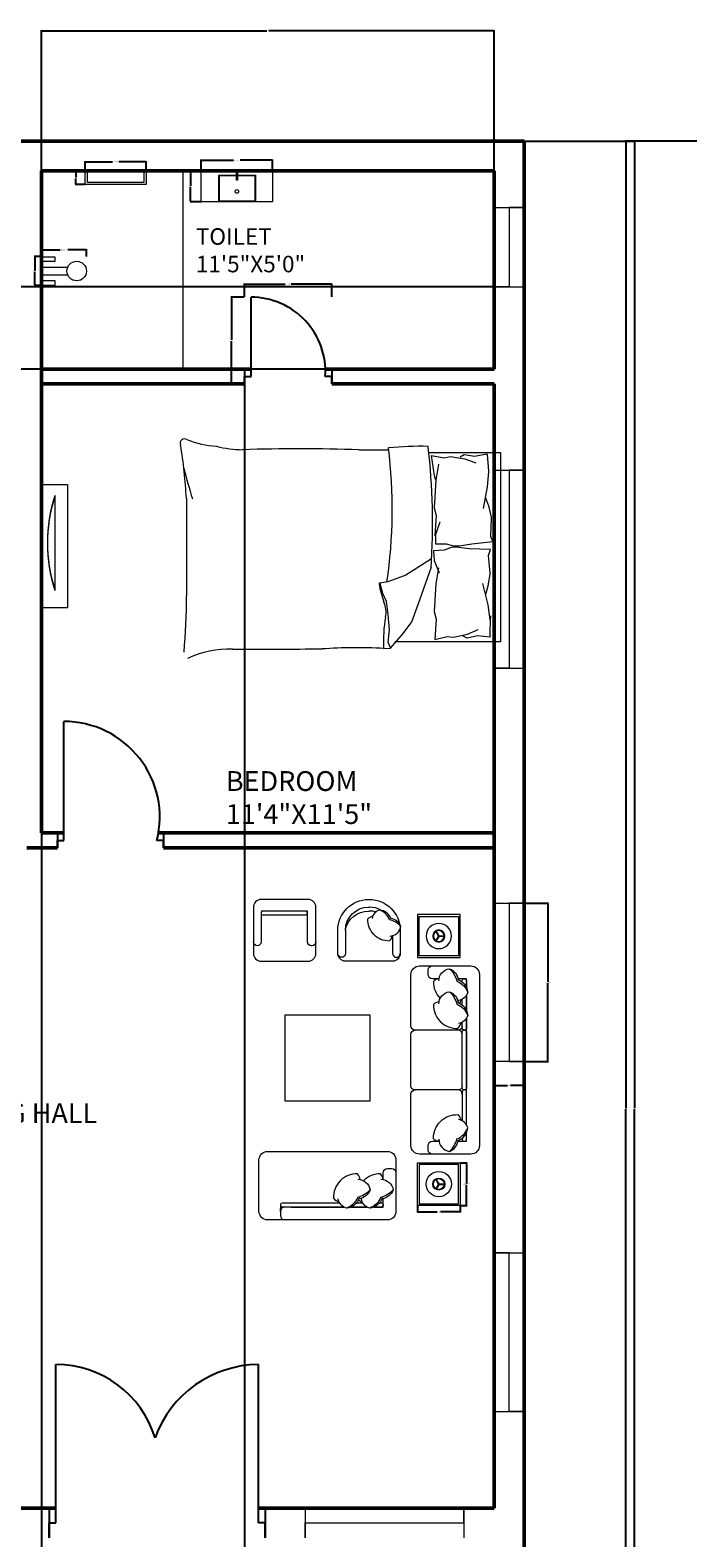
# Model space of a CAD drawing. Units: inches. Extents: x 2268 to 3372, y 1709 to 2892.
# Tile 3 of 6: x 2563 to 2762, y 2040 to 2497. Entities that reach past the tile are written whole.
import ezdxf

# ---------------------------------------------------------------- set-up
doc = ezdxf.new("R2010")
doc.units = ezdxf.units.IN
for name, color, linetype, lineweight in [('A-ANNO-DIMS', 2, 'Continuous', 18), ('A-AREA-IDEN', 7, 'Continuous', 18), ('A-DOOR', 3, 'Continuous', 25), ('A-FLOR-FIXT', 9, 'Continuous', 18), ('A-FURN', 8, 'Continuous', 18), ('A-GLAZ', 4, 'Continuous', 18), ('A-WALL', 7, 'Continuous', 50)]:
    doc.layers.add(name, color=color, linetype=linetype, lineweight=lineweight)
doc.styles.get("Standard").update_dxf_attribs({"font": 'arial.ttf'})
doc.dimstyles.get("Standard").update_dxf_attribs({"dimtxt": 0.18, "dimasz": 0.18, "dimexe": 0.18, "dimexo": 0.0625, "dimgap": 0.09, "dimtad": 0, "dimtih": 1, "dimtoh": 1, "dimdec": 4, "dimzin": 0, "dimdsep": 46, "dimtxsty": 'Standard', "dimcen": 0.09, "dimadec": 0, "dimazin": 0, "dimtfac": 1, "dimtdec": 4, "dimtofl": 0, "dimtmove": 0, "dimatfit": 3, "dimfxl": 1, "dimtolj": 1, "dimtzin": 0, "dimarcsym": 0})

# ---------------------------------------------------------------- blocks, each defined once
blk = doc.blocks.new('DOOR-ENTRY-PAIR')
for p, q in [((2, 4.5), (2, 52.5)), ((63.28, 40.5), (63.28, 52.5)), ((63.28, 4.5), (63.28, 40.5)), ((0, 9), (0, 0)), ((65.28, 9), (65.28, 0)), ((0, 0), (0, 4.5)), ((0, 4.5), (2, 4.5)), ((65.28, 4.5), (63.28, 4.5)), ((65.28, 0), (65.28, 4.5))]:
    blk.add_line(p, q)
for centre, radius, start, end in [((2, 21.15), 31.35, 16.9315, 90), ((63.59, 18.92), 33.58, 90.5202, 160.2273)]:
    blk.add_arc(centre, radius, start, end)
blk = doc.blocks.new('DOOR-BEDROOM-E')
for p, q in [((2, 2.25), (2, 38.25)), ((0, 4.5), (0, 0)), ((0, 0), (0, 2.25)), ((0, 2.25), (2, 2.25)), ((32.14, 2.25), (30.14, 2.25)), ((32.14, 4.5), (32.14, 0)), ((32.14, 0), (32.14, 2.25))]:
    blk.add_line(p, q)
blk.add_arc((2, 9.25), 29, 346.0304, 90)
blk = doc.blocks.new('DOOR-BATH-E')
for p, q in [((2, 2.25), (2, 26.25)), ((0, 4.5), (0, 0)), ((0, 0), (0, 2.25)), ((0, 2.25), (2, 2.25)), ((26.44, 2.25), (24.44, 2.25)), ((26.44, 4.5), (26.44, 0)), ((26.44, 0), (26.44, 2.25))]:
    blk.add_line(p, q)
blk.add_arc((2, 3.76), 22.49, 356.1476, 90)
blk = doc.blocks.new('WIN-48')
for p, q in [((0, 9), (0, 0)), ((48, 4.5), (48, 9)), ((48, 9), (48, 0)), ((0, 0), (0, 4.5)), ((0, 4.5), (48, 4.5))]:
    blk.add_line(p, q)
blk = doc.blocks.new('WIN-24-LONGITUDINAL')
for p, q in [((0, 24), (9, 24)), ((9, 24), (4.5, 24)), ((4.5, 24), (4.5, 0)), ((4.5, 0), (0, 0)), ((0, 0), (9, 0))]:
    blk.add_line(p, q)
blk = doc.blocks.new('WIN-60-ALTERNATE')
for p, q in [((0, 60), (9, 60)), ((9, 60), (4.5, 60)), ((4.5, 60), (4.5, 0)), ((4.5, 0), (0, 0)), ((0, 0), (9, 0))]:
    blk.add_line(p, q)
blk = doc.blocks.new('WIN-48-ALTERNATE')
for p, q in [((0, 48), (9, 48)), ((9, 48), (4.5, 48)), ((4.5, 48), (4.5, 0)), ((9, 0), (0, 0)), ((4.5, 0), (9, 0))]:
    blk.add_line(p, q)
blk = doc.blocks.new('LAVATORY-VANITY')
for points in [[(0, 9.35), (21.53, 9.35), (21.53, 0), (0, 0)], [(10.67, 8.74), (11.01, 8.74), (11.01, 6.59), (10.67, 6.59)]]:
    blk.add_lwpolyline(points, close=True)
for points in [[(11.01, 8.1), (16.38, 8.1), (16.38, 0), (5.34, 0), (5.34, 8.1), (10.67, 8.1)], [(11.01, 7.98), (16.25, 7.98), (16.25, 0.14), (5.47, 0.14), (5.47, 7.98), (10.67, 7.98)]]:
    blk.add_lwpolyline(points)
blk.add_circle((10.78, 3.14), 0.562)
blk = doc.blocks.new('SHOWER-FITTING')
for points in [[(0, 8.74), (4.04, 8.74), (4.04, 7.26), (0, 7.26)], [(0, 1.48), (4.04, 1.48), (4.04, 0), (0, 0)]]:
    blk.add_lwpolyline(points, close=True)
blk.add_lwpolyline([(7.94, 3.17), (0, 3.17), (0, 5.6), (7.94, 5.6)])
blk.add_circle((10.64, 4.38), 2.96)
blk = doc.blocks.new('SHOWER-SHELF')
for points in [[(0, 4.16), (18.51, 4.16), (18.51, 0), (0, 0)], [(0.76, 4.16), (17.78, 4.16), (17.78, 0.69), (0.76, 0.69)]]:
    blk.add_lwpolyline(points, close=True)
blk = doc.blocks.new('BEDROOM-WALL-UNIT-E')
for p, q in [((4.02, 34.02), (4.02, 5.6)), ((4.02, 33.67), (4.02, 5.25))]:
    blk.add_line(p, q)
blk.add_lwpolyline([(0, 37.37), (7.87, 37.37), (7.87, 0), (0, 0)], close=True)
for centre in [(47.85, 19.81), (47.85, 19.46)]:
    blk.add_arc(centre, 46.08, 162.0375, 197.9625)
blk = doc.blocks.new('BED-DOUBLE')
for p, q in [((0, 61.46), (31.9, 61.46)), ((0, 4.17), (0, 61.46)), ((1.84, 4.17), (1.84, 61.46)), ((3.07, 60.08), (2.95, 53.6)), ((3.07, 60.08), (6.92, 59.62)), ((6.92, 59.62), (10, 60.34)), ((14.18, 60.08), (9.9, 59.11)), ((10, 60.34), (11.25, 59.72)), ((16.11, 59.85), (14.18, 60.08)), ((19.87, 60.78), (16.11, 59.85)), ((19.38, 54.63), (19.87, 60.78)), ((33.26, 63.38), (29.37, 58.94)), ((35.36, 63.48), (33.26, 63.38, 4.64)), ((34.01, 61.54), (33.26, 63.38)), ((33.63, 57.82), (34.01, 61.54)), ((2.95, 53.6), (3.05, 54.8)), ((3.05, 54.8), (3.68, 50.25)), ((9.9, 59.11), (6.69, 57.7)), ((26.77, 55.41), (24.36, 48.73)), ((29.37, 58.94), (26.77, 55.41)), ((34.01, 53.18), (33.63, 57.82)), ((3.68, 50.25), (5.3, 43.75)), ((20.05, 52.28), (19.38, 54.63)), ((19.54, 43.87), (20.05, 52.28)), ((34.56, 49.1), (34.01, 53.18)), ((4.4, 47), (3.69, 44.52)), ((24.36, 48.73), (20.84, 38.73)), ((35.68, 46.68), (34.56, 49.1)), ((36.42, 43.71), (35.68, 46.68)), ((95, 18.06), (95, 47.57)), ((3.69, 44.52), (3.04, 41.01)), ((18.74, 39.04), (19.54, 43.87)), ((20.84, 36.28), (28.62, 41.3)), ((28.62, 41.3), (34.01, 43.34)), ((34.01, 43.34), (36.42, 43.71)), ((3.04, 41.01), (3.07, 40.62)), ((3.07, 40.62), (3.57, 35.31)), ((20.07, 36.86), (18.53, 40.55)), ((20.25, 33.92), (20.07, 36.86)), ((3.57, 35.31), (2.99, 33.54)), ((2.99, 33.54), (9.43, 33.25)), ((8.66, 31.84), (12.47, 32.54)), ((9.43, 33.25), (13.28, 32.79)), ((12.47, 32.54), (14.03, 32.54)), ((13.28, 32.79), (14.84, 32.89)), ((14.03, 32.54), (16.28, 31.84)), ((14.84, 32.89), (17.04, 33.72)), ((17.04, 33.72), (20.25, 33.92)), ((2.24, 31.15), (8.66, 31.84)), ((2.94, 29.42), (2.24, 31.15)), ((2.76, 24.09), (2.94, 29.42)), ((16.28, 31.84), (19.5, 31.84)), ((19.5, 28.9), (18.19, 25.13)), ((19.38, 23.24), (19.87, 29.39)), ((19.5, 31.84), (19.5, 28.9)), ((2.76, 23.7), (2.76, 24.09)), ((3.63, 20.23), (2.76, 23.7)), ((20.05, 20.89), (19.38, 23.24)), ((4.5, 17.81), (3.63, 20.23)), ((3.98, 14.52), (5.19, 21.1)), ((19.54, 12.48), (20.05, 20.89)), ((3.63, 9.93), (3.98, 14.52)), ((3.61, 9.81), (3.63, 9.93)), ((4, 4.67), (3.61, 9.81)), ((18.74, 7.65), (19.54, 12.48)), ((19.54, 12.48), (19.92, 11.13)), ((19.92, 11.13), (20.79, 5.02)), ((3.98, 4.67), (7.79, 5.36)), ((10.74, 6.06), (7.44, 7.27)), ((7.79, 5.36), (10.91, 4.84)), ((15.07, 5.36), (10.74, 6.06)), ((10.91, 4.84), (12.12, 5.54)), ((16.98, 5.71), (15.07, 5.36)), ((20.79, 5.02), (16.98, 5.71)), ((21.71, 4.17), (0, 4.17))]:
    blk.add_line(p, q)
for centre, radius, start, end in [((82.32, 91.3), 27.65, 267.4714, 296.4681), ((254.49, 49.33), 159.5, 174.4998, 180.6351), ((-7.98, 61.53), 43.38, 349.8763, 2.5657), ((43.54, 218.51), 155.25, 266.9791, 273.8365), ((81.31, -5405.34), 5469.02, 90.00217, 90.28689), ((42.04, 52.44), 7.46, 168.6608, 203.7384), ((1.78, 37.35), 35.55, 10.6617, 19.8806), ((187.4, 21.29), 154.68, 171.7845, 186.9006), ((36.49, 43.92), 0.221, 250.2464, 1.1377), ((218.26, 25.61), 197.77, 176.0865, 186.7821), ((-28.43, -20.65), 127.63, 13.3832, 17.7053), ((240.78, 25.69), 145.97, 182.9958, 189.4091), ((24.09, 102.1), 99.87, 268.7218, 275.604), ((37.37, -200.58), 203.94, 88.4762, 91.0082), ((60.68, 581.23), 578.22, 268.22771, 271.71854), ((77.34, -32.25), 35.53, 76.0648, 88.9113), ((84.25, -25.97), 28.25, 67.9751, 86.652), ((95.57, 1.3), 1.31, 236.1736, 23.4781)]:
    blk.add_arc(centre, radius, start, end)
blk = doc.blocks.new('LIVING-END-TABLE')
for p, q in [((6.41, 6.44), (5.49, 8.02)), ((6.41, 6.52), (5.49, 4.94)), ((6.55, 6.52), (5.63, 8.1)), ((6.55, 6.44), (5.63, 4.85)), ((6.48, 6.56), (8.3, 6.56)), ((6.48, 6.39), (8.3, 6.39))]:
    blk.add_line(p, q)
at = {"ltscale": 0.03}
blk.add_lwpolyline([(0, 0), (0, 12.95), (12.95, 12.95), (12.95, 0)], close=True, dxfattribs=at)
blk.add_lwpolyline([(0.52, 12.43), (0.52, 0.52), (12.43, 0.52), (12.43, 12.43)], close=True)
for radius in [3.82, 1.83, 1.64]:
    blk.add_circle((6.48, 6.48), radius)
blk = doc.blocks.new('*D38')
at = {"layer": 'A-ANNO-DIMS', "color": 0, "lineweight": -2, "transparency": 16777216}
for p, q in [((2628.3, 2415.99), (2628.3, 2420.07)), ((2628.48, 2419.89), (2640.59, 2419.89)), ((2654.56, 2419.89), (2642.46, 2419.89)), ((2654.74, 2415.99), (2654.74, 2420.07))]:
    blk.add_line(p, q, dxfattribs=at)
at = {"layer": 'A-ANNO-DIMS', "color": 0, "transparency": 16777216}
for points in [[(2628.48, 2419.92), (2628.48, 2419.86), (2628.3, 2419.89)], [(2654.56, 2419.92), (2654.56, 2419.86), (2654.74, 2419.89)]]:
    blk.add_solid(points, dxfattribs=at)
at = {"layer": 'Defpoints', "color": 0, "transparency": 16777216}
for p in [(2628.3, 2415.93), (2654.74, 2419.89), (2654.74, 2415.93)]:
    blk.add_point(p, dxfattribs=at)
at = {"layer": 'A-ANNO-DIMS', "color": 0, "transparency": 16777216, "insert": (2641.52, 2419.89), "char_height": 0.18, "attachment_point": 5}
blk.add_mtext('\\A1;DOOR 26 TYP.', dxfattribs=at)
blk = doc.blocks.new('*D39')
at = {"layer": 'A-ANNO-DIMS', "color": 0, "lineweight": -2, "transparency": 16777216}
for p, q in [((2628.24, 2415.93), (2624.16, 2415.93)), ((2624.34, 2415.75), (2624.34, 2402.98)), ((2624.34, 2389.86), (2624.34, 2402.62)), ((2628.24, 2389.68), (2624.16, 2389.68))]:
    blk.add_line(p, q, dxfattribs=at)
at = {"layer": 'A-ANNO-DIMS', "color": 0, "transparency": 16777216}
for points in [[(2624.31, 2415.75), (2624.37, 2415.75), (2624.34, 2415.93)], [(2624.31, 2389.86), (2624.37, 2389.86), (2624.34, 2389.68)]]:
    blk.add_solid(points, dxfattribs=at)
at = {"layer": 'Defpoints', "color": 0, "transparency": 16777216}
for p in [(2624.34, 2415.93), (2628.3, 2415.93), (2628.3, 2389.68)]:
    blk.add_point(p, dxfattribs=at)
at = {"layer": 'A-ANNO-DIMS', "color": 0, "transparency": 16777216, "insert": (2624.34, 2402.8), "char_height": 0.18, "attachment_point": 5}
blk.add_mtext('\\A1;26 TYP.', dxfattribs=at)
blk = doc.blocks.new('*D54')
at = {"layer": 'A-ANNO-DIMS', "color": 0, "lineweight": -2, "transparency": 16777216}
for p, q in [((2712.96, 2232.4), (2720.27, 2232.4)), ((2720.09, 2232.22), (2720.09, 2208.59)), ((2720.09, 2184.58), (2720.09, 2208.22)), ((2712.96, 2184.4), (2720.27, 2184.4))]:
    blk.add_line(p, q, dxfattribs=at)
at = {"layer": 'A-ANNO-DIMS', "color": 0, "transparency": 16777216}
for points in [[(2720.06, 2232.22), (2720.12, 2232.22), (2720.09, 2232.4)], [(2720.06, 2184.58), (2720.12, 2184.58), (2720.09, 2184.4)]]:
    blk.add_solid(points, dxfattribs=at)
at = {"layer": 'Defpoints', "color": 0, "transparency": 16777216}
for p in [(2712.89, 2232.4), (2720.09, 2232.4), (2712.89, 2184.4)]:
    blk.add_point(p, dxfattribs=at)
at = {"layer": 'A-ANNO-DIMS', "color": 0, "transparency": 16777216, "insert": (2720.09, 2208.4), "char_height": 0.18, "attachment_point": 5}
blk.add_mtext('\\A1;WINDOW 48 TYP.', dxfattribs=at)
blk = doc.blocks.new('*D55')
at = {"layer": 'A-ANNO-DIMS', "color": 0, "lineweight": -2, "transparency": 16777216}
for p, q in [((2703.89, 2184.34), (2703.89, 2177.02)), ((2712.89, 2184.34), (2712.89, 2177.02)), ((2704.07, 2177.2), (2707.94, 2177.2)), ((2712.71, 2177.2), (2708.85, 2177.2))]:
    blk.add_line(p, q, dxfattribs=at)
at = {"layer": 'A-ANNO-DIMS', "color": 0, "transparency": 16777216}
for points in [[(2704.07, 2177.23), (2704.07, 2177.17), (2703.89, 2177.2)], [(2712.71, 2177.23), (2712.71, 2177.17), (2712.89, 2177.2)]]:
    blk.add_solid(points, dxfattribs=at)
at = {"layer": 'Defpoints', "color": 0, "transparency": 16777216}
for p in [(2703.89, 2184.4), (2712.89, 2184.4), (2712.89, 2177.2)]:
    blk.add_point(p, dxfattribs=at)
at = {"layer": 'A-ANNO-DIMS', "color": 0, "transparency": 16777216, "insert": (2708.39, 2177.2), "char_height": 0.18, "attachment_point": 5}
blk.add_mtext('\\A1;9 TYP.', dxfattribs=at)
blk = doc.blocks.new('*D60')
at = {"layer": 'A-ANNO-DIMS', "color": 0, "lineweight": -2, "transparency": 16777216}
for p, q in [((2615.23, 2454.24), (2615.23, 2457.59)), ((2615.41, 2457.41), (2624.97, 2457.41)), ((2636.58, 2457.41), (2627.01, 2457.41)), ((2636.76, 2454.24), (2636.76, 2457.59))]:
    blk.add_line(p, q, dxfattribs=at)
at = {"layer": 'A-ANNO-DIMS', "color": 0, "transparency": 16777216}
for points in [[(2615.41, 2457.44), (2615.41, 2457.38), (2615.23, 2457.41)], [(2636.58, 2457.44), (2636.58, 2457.38), (2636.76, 2457.41)]]:
    blk.add_solid(points, dxfattribs=at)
at = {"layer": 'Defpoints', "color": 0, "transparency": 16777216}
for p in [(2636.76, 2457.41), (2615.23, 2454.18), (2636.76, 2454.18)]:
    blk.add_point(p, dxfattribs=at)
at = {"layer": 'A-ANNO-DIMS', "color": 0, "transparency": 16777216, "insert": (2625.99, 2457.41), "char_height": 0.18, "attachment_point": 5}
blk.add_mtext('\\A1;VANITY 22 TYP.', dxfattribs=at)
blk = doc.blocks.new('*D61')
at = {"layer": 'A-ANNO-DIMS', "color": 0, "lineweight": -2, "transparency": 16777216}
for p, q in [((2615.16, 2454.18), (2611.82, 2454.18)), ((2612, 2454), (2612, 2449.68)), ((2612, 2445), (2612, 2449.32)), ((2615.16, 2444.82), (2611.82, 2444.82))]:
    blk.add_line(p, q, dxfattribs=at)
at = {"layer": 'A-ANNO-DIMS', "color": 0, "transparency": 16777216}
for points in [[(2611.97, 2454), (2612.03, 2454), (2612, 2454.18)], [(2611.97, 2445), (2612.03, 2445), (2612, 2444.82)]]:
    blk.add_solid(points, dxfattribs=at)
at = {"layer": 'Defpoints', "color": 0, "transparency": 16777216}
for p in [(2612, 2454.18), (2615.23, 2454.18), (2615.23, 2444.82)]:
    blk.add_point(p, dxfattribs=at)
at = {"layer": 'A-ANNO-DIMS', "color": 0, "transparency": 16777216, "insert": (2612, 2449.5), "char_height": 0.18, "attachment_point": 5}
blk.add_mtext('\\A1;9 TYP.', dxfattribs=at)
blk = doc.blocks.new('*D62')
at = {"layer": 'A-ANNO-DIMS', "color": 0, "lineweight": -2, "transparency": 16777216}
for p, q in [((2566.89, 2428.27), (2566.89, 2430.43)), ((2567.07, 2430.25), (2572.57, 2430.25)), ((2580.32, 2430.25), (2574.82, 2430.25)), ((2580.5, 2428.27), (2580.5, 2430.43))]:
    blk.add_line(p, q, dxfattribs=at)
at = {"layer": 'A-ANNO-DIMS', "color": 0, "transparency": 16777216}
for points in [[(2567.07, 2430.28), (2567.07, 2430.22), (2566.89, 2430.25)], [(2580.32, 2430.28), (2580.32, 2430.22), (2580.5, 2430.25)]]:
    blk.add_solid(points, dxfattribs=at)
at = {"layer": 'Defpoints', "color": 0, "transparency": 16777216}
for p in [(2580.5, 2430.25), (2566.89, 2428.21), (2580.5, 2428.21)]:
    blk.add_point(p, dxfattribs=at)
at = {"layer": 'A-ANNO-DIMS', "color": 0, "transparency": 16777216, "insert": (2573.7, 2430.25), "char_height": 0.18, "attachment_point": 5}
blk.add_mtext('\\A1;SHOWER 14 TYP.', dxfattribs=at)
blk = doc.blocks.new('*D63')
at = {"layer": 'A-ANNO-DIMS', "color": 0, "lineweight": -2, "transparency": 16777216}
for p, q in [((2566.83, 2428.21), (2564.67, 2428.21)), ((2564.85, 2428.03), (2564.85, 2424.02)), ((2564.85, 2419.64), (2564.85, 2423.65)), ((2566.83, 2419.46), (2564.67, 2419.46))]:
    blk.add_line(p, q, dxfattribs=at)
at = {"layer": 'A-ANNO-DIMS', "color": 0, "transparency": 16777216}
for points in [[(2564.82, 2428.03), (2564.88, 2428.03), (2564.85, 2428.21)], [(2564.82, 2419.64), (2564.88, 2419.64), (2564.85, 2419.46)]]:
    blk.add_solid(points, dxfattribs=at)
at = {"layer": 'Defpoints', "color": 0, "transparency": 16777216}
for p in [(2564.85, 2428.21), (2566.89, 2428.21), (2566.89, 2419.46)]:
    blk.add_point(p, dxfattribs=at)
at = {"layer": 'A-ANNO-DIMS', "color": 0, "transparency": 16777216, "insert": (2564.85, 2423.83), "char_height": 0.18, "attachment_point": 5}
blk.add_mtext('\\A1;9 TYP.', dxfattribs=at)
blk = doc.blocks.new('*D64')
at = {"layer": 'A-ANNO-DIMS', "color": 0, "lineweight": -2, "transparency": 16777216}
for p, q in [((2580.05, 2454.24), (2580.05, 2457.13)), ((2580.23, 2456.95), (2588.34, 2456.95)), ((2598.39, 2456.95), (2590.28, 2456.95)), ((2598.57, 2454.24), (2598.57, 2457.13))]:
    blk.add_line(p, q, dxfattribs=at)
at = {"layer": 'A-ANNO-DIMS', "color": 0, "transparency": 16777216}
for points in [[(2580.23, 2456.98), (2580.23, 2456.92), (2580.05, 2456.95)], [(2598.39, 2456.98), (2598.39, 2456.92), (2598.57, 2456.95)]]:
    blk.add_solid(points, dxfattribs=at)
at = {"layer": 'Defpoints', "color": 0, "transparency": 16777216}
for p in [(2598.57, 2456.95), (2580.05, 2454.18), (2598.57, 2454.18)]:
    blk.add_point(p, dxfattribs=at)
at = {"layer": 'A-ANNO-DIMS', "color": 0, "transparency": 16777216, "insert": (2589.31, 2456.95), "char_height": 0.18, "attachment_point": 5}
blk.add_mtext('\\A1;SHELF 19 TYP.', dxfattribs=at)
blk = doc.blocks.new('*D65')
at = {"layer": 'A-ANNO-DIMS', "color": 0, "lineweight": -2, "transparency": 16777216}
for p, q in [((2579.99, 2454.18), (2577.09, 2454.18)), ((2577.27, 2454), (2577.27, 2452.28)), ((2579.99, 2450.02), (2577.09, 2450.02)), ((2577.27, 2450.2), (2577.27, 2451.92))]:
    blk.add_line(p, q, dxfattribs=at)
at = {"layer": 'A-ANNO-DIMS', "color": 0, "transparency": 16777216}
for points in [[(2577.24, 2454), (2577.3, 2454), (2577.27, 2454.18)], [(2577.24, 2450.2), (2577.3, 2450.2), (2577.27, 2450.02)]]:
    blk.add_solid(points, dxfattribs=at)
at = {"layer": 'Defpoints', "color": 0, "transparency": 16777216}
for p in [(2577.27, 2454.18), (2580.05, 2454.18), (2580.05, 2450.02)]:
    blk.add_point(p, dxfattribs=at)
at = {"layer": 'A-ANNO-DIMS', "color": 0, "transparency": 16777216, "insert": (2577.27, 2452.1), "char_height": 0.18, "attachment_point": 5}
blk.add_mtext('\\A1;4 TYP.', dxfattribs=at)
blk = doc.blocks.new('*D72')
at = {"layer": 'A-ANNO-DIMS', "color": 0, "lineweight": -2, "transparency": 16777216}
for p, q in [((2693.64, 2153.8), (2695.7, 2153.8)), ((2695.52, 2153.62), (2695.52, 2147.5)), ((2695.52, 2141.02), (2695.52, 2147.14)), ((2693.64, 2140.84), (2695.7, 2140.84))]:
    blk.add_line(p, q, dxfattribs=at)
at = {"layer": 'A-ANNO-DIMS', "color": 0, "transparency": 16777216}
for points in [[(2695.49, 2153.62), (2695.55, 2153.62), (2695.52, 2153.8)], [(2695.49, 2141.02), (2695.55, 2141.02), (2695.52, 2140.84)]]:
    blk.add_solid(points, dxfattribs=at)
at = {"layer": 'Defpoints', "color": 0, "transparency": 16777216}
for p in [(2693.58, 2153.8), (2695.52, 2153.8), (2693.58, 2140.84)]:
    blk.add_point(p, dxfattribs=at)
at = {"layer": 'A-ANNO-DIMS', "color": 0, "transparency": 16777216, "insert": (2695.52, 2147.32), "char_height": 0.18, "attachment_point": 5}
blk.add_mtext('\\A1;END TABLE 13 TYP.', dxfattribs=at)
blk = doc.blocks.new('*D73')
at = {"layer": 'A-ANNO-DIMS', "color": 0, "lineweight": -2, "transparency": 16777216}
for p, q in [((2680.63, 2140.78), (2680.63, 2138.72)), ((2680.81, 2138.9), (2686.58, 2138.9)), ((2693.4, 2138.9), (2687.62, 2138.9)), ((2693.58, 2140.78), (2693.58, 2138.72))]:
    blk.add_line(p, q, dxfattribs=at)
at = {"layer": 'A-ANNO-DIMS', "color": 0, "transparency": 16777216}
for points in [[(2680.81, 2138.93), (2680.81, 2138.87), (2680.63, 2138.9)], [(2693.4, 2138.93), (2693.4, 2138.87), (2693.58, 2138.9)]]:
    blk.add_solid(points, dxfattribs=at)
at = {"layer": 'Defpoints', "color": 0, "transparency": 16777216}
for p in [(2680.63, 2140.84), (2693.58, 2140.84), (2693.58, 2138.9)]:
    blk.add_point(p, dxfattribs=at)
at = {"layer": 'A-ANNO-DIMS', "color": 0, "transparency": 16777216, "insert": (2687.1, 2138.9), "char_height": 0.18, "attachment_point": 5}
blk.add_mtext('\\A1;13 TYP.', dxfattribs=at)
blk = doc.blocks.new('*D77')
at = {"layer": 'A-ANNO-DIMS', "color": 0, "lineweight": -2, "transparency": 16777216}
for p, q in [((2712.96, 2463.18), (2746.52, 2463.18)), ((2746.34, 2463), (2746.34, 2170.36)), ((2746.34, 1877.36), (2746.34, 2169.99)), ((2712.96, 1877.18), (2746.52, 1877.18))]:
    blk.add_line(p, q, dxfattribs=at)
at = {"layer": 'A-ANNO-DIMS', "color": 0, "transparency": 16777216}
for points in [[(2746.31, 2463), (2746.37, 2463), (2746.34, 2463.18)], [(2746.31, 1877.36), (2746.37, 1877.36), (2746.34, 1877.18)]]:
    blk.add_solid(points, dxfattribs=at)
at = {"layer": 'Defpoints', "color": 0, "transparency": 16777216}
for p in [(2712.89, 2463.18), (2746.34, 2463.18), (2712.89, 1877.18)]:
    blk.add_point(p, dxfattribs=at)
at = {"layer": 'A-ANNO-DIMS', "color": 0, "transparency": 16777216, "insert": (2746.34, 2170.18), "char_height": 0.18, "attachment_point": 5}
blk.add_mtext('\\A1;586', dxfattribs=at)
blk = doc.blocks.new('*D80')
at = {"layer": 'A-ANNO-DIMS', "color": 0, "lineweight": -2, "transparency": 16777216}
for p, q in [((2566.89, 2454.24), (2566.89, 2496.81)), ((2567.07, 2496.63), (2635.11, 2496.63)), ((2703.71, 2496.63), (2635.67, 2496.63)), ((2703.89, 2454.24), (2703.89, 2496.81))]:
    blk.add_line(p, q, dxfattribs=at)
at = {"layer": 'A-ANNO-DIMS', "color": 0, "transparency": 16777216}
for points in [[(2567.07, 2496.66), (2567.07, 2496.6), (2566.89, 2496.63)], [(2703.71, 2496.66), (2703.71, 2496.6), (2703.89, 2496.63)]]:
    blk.add_solid(points, dxfattribs=at)
at = {"layer": 'Defpoints', "color": 0, "transparency": 16777216}
for p in [(2703.89, 2496.63), (2566.89, 2454.18), (2703.89, 2454.18)]:
    blk.add_point(p, dxfattribs=at)
at = {"layer": 'A-ANNO-DIMS', "color": 0, "transparency": 16777216, "insert": (2635.39, 2496.63), "char_height": 0.18, "attachment_point": 5}
blk.add_mtext('\\A1;137', dxfattribs=at)
blk = doc.blocks.new('*D82')
at = {"layer": 'A-ANNO-DIMS', "color": 0, "lineweight": -2, "transparency": 16777216}
for p, q in [((2566.89, 2389.61), (2566.89, 1790.27)), ((2628.3, 2389.61), (2628.3, 1790.27)), ((2567.07, 1790.45), (2597.22, 1790.45)), ((2628.12, 1790.45), (2597.98, 1790.45))]:
    blk.add_line(p, q, dxfattribs=at)
at = {"layer": 'A-ANNO-DIMS', "color": 0, "transparency": 16777216}
for points in [[(2567.07, 1790.48), (2567.07, 1790.42), (2566.89, 1790.45)], [(2628.12, 1790.48), (2628.12, 1790.42), (2628.3, 1790.45)]]:
    blk.add_solid(points, dxfattribs=at)
at = {"layer": 'Defpoints', "color": 0, "transparency": 16777216}
for p in [(2566.89, 2389.68), (2628.3, 2389.68), (2628.3, 1790.45)]:
    blk.add_point(p, dxfattribs=at)
at = {"layer": 'A-ANNO-DIMS', "color": 0, "transparency": 16777216, "insert": (2597.6, 1790.45), "char_height": 0.18, "attachment_point": 5}
blk.add_mtext('\\A1;61.41', dxfattribs=at)
blk = doc.blocks.new('*D93')
at = {"layer": 'A-ANNO-DIMS', "color": 0, "lineweight": -2, "transparency": 16777216}
for p, q in [((2812.94, 2463.18), (2743.52, 2463.18)), ((2743.7, 2463), (2743.7, 2170.36)), ((2743.7, 1877.36), (2743.7, 2169.99)), ((2812.94, 1877.18), (2743.52, 1877.18))]:
    blk.add_line(p, q, dxfattribs=at)
at = {"layer": 'A-ANNO-DIMS', "color": 0, "transparency": 16777216}
for points in [[(2743.67, 2463), (2743.73, 2463), (2743.7, 2463.18)], [(2743.67, 1877.36), (2743.73, 1877.36), (2743.7, 1877.18)]]:
    blk.add_solid(points, dxfattribs=at)
at = {"layer": 'Defpoints', "color": 0, "transparency": 16777216}
for p in [(2743.7, 2463.18), (2813, 2463.18), (2813, 1877.18)]:
    blk.add_point(p, dxfattribs=at)
at = {"layer": 'A-ANNO-DIMS', "color": 0, "transparency": 16777216, "insert": (2743.7, 2170.18), "char_height": 0.18, "attachment_point": 5}
blk.add_mtext('\\A1;586', dxfattribs=at)
blk = doc.blocks.new('*D98')
at = {"layer": 'A-ANNO-DIMS', "color": 0, "lineweight": -2, "transparency": 16777216}
for p, q in [((2703.83, 2419.05), (2329.26, 2419.05)), ((2329.44, 2418.87), (2329.44, 2406.8)), ((2329.44, 2394.36), (2329.44, 2406.43)), ((2703.83, 2394.18), (2329.26, 2394.18))]:
    blk.add_line(p, q, dxfattribs=at)
at = {"layer": 'A-ANNO-DIMS', "color": 0, "transparency": 16777216}
for points in [[(2329.41, 2418.87), (2329.47, 2418.87), (2329.44, 2419.05)], [(2329.41, 2394.36), (2329.47, 2394.36), (2329.44, 2394.18)]]:
    blk.add_solid(points, dxfattribs=at)
at = {"layer": 'Defpoints', "color": 0, "transparency": 16777216}
for p in [(2329.44, 2419.05), (2703.89, 2419.05), (2703.89, 2394.18)]:
    blk.add_point(p, dxfattribs=at)
at = {"layer": 'A-ANNO-DIMS', "color": 0, "transparency": 16777216, "insert": (2329.44, 2406.61), "char_height": 0.18, "attachment_point": 5}
blk.add_mtext('\\A1;24.88', dxfattribs=at)

msp = doc.modelspace()

# ---------------------------------------------------------------- linework, layer by layer
at = {"layer": 'A-FLOR-FIXT'}
msp.add_line((2609.6995, 2454.1756), (2609.6995, 2394.1756), dxfattribs=at)
msp.add_line((2609.6995, 2454.1756), (2609.6995, 2394.1756), dxfattribs=at)
at = {"layer": 'A-FURN'}
msp.add_line((2639.1743, 2139.0646), (2639.3001, 2141.0076), dxfattribs=at)
at = {"layer": 'A-FURN', "ltscale": 0.03}
for points in [[(2633.3396, 2233.5207), (2633.3396, 2233.5207, 0.41421356), (2631.0037, 2231.1848), (2631.0037, 2217.1696, 0.41421356), (2633.3396, 2214.8337), (2633.3396, 2214.8337), (2647.5885, 2214.8337, 0.41421356), (2649.9244, 2217.1696), (2649.9244, 2231.1848, 0.41421356), (2647.5885, 2233.5207)], [(2681.2733, 2156.3858, -0.41421356), (2678.6826, 2158.9765), (2678.6826, 2174.5207, -0.41421356), (2679.9779, 2175.816, -0.41421356), (2678.6826, 2177.1114), (2678.6826, 2192.6556, -0.41421356), (2679.9779, 2193.951, -0.41421356), (2678.6826, 2195.2463), (2678.6826, 2210.7905, -0.41421356), (2681.2733, 2213.3812), (2696.8175, 2213.3812, -0.41421356), (2699.4082, 2210.7905), (2699.4082, 2158.9765, -0.41421356), (2696.8175, 2156.3858)], [(2632.6976, 2154.6088, -0.41421356), (2635.2883, 2157.1995), (2635.2883, 2157.1995, 0.31783725), (2635.2883, 2157.1995, -0.41421356), (2635.2883, 2157.1995), (2635.2883, 2157.1995, 1.18618475), (2635.2883, 2157.1995, -0.41421356), (2635.2883, 2157.1995), (2671.5581, 2157.1995, -0.41421356), (2674.1488, 2154.6088), (2674.1488, 2139.0646, -0.41421356), (2671.5581, 2136.4739), (2635.2883, 2136.4739, -0.41421356), (2632.6976, 2139.0646)]]:
    msp.add_lwpolyline(points, format="xyb", close=True, dxfattribs=at)
msp.add_lwpolyline([(2665.9881, 2214.8337), (2658.8637, 2214.8337, -0.41421356), (2656.5278, 2217.1696), (2656.5278, 2224.1772, -0.41421356), (2665.8713, 2233.5207), (2665.9881, 2233.5207), (2666.1049, 2233.5207, -0.41421356), (2675.4484, 2224.1772), (2675.4484, 2217.1696, -0.41421356), (2673.1126, 2214.8337), (2665.9881, 2214.8337)], format="xyb", dxfattribs=at)
at = {"layer": 'A-FURN'}
for points in [[(2633.3396, 2229.3161), (2633.3396, 2220.6734, -0.41421356), (2632.1717, 2219.5054), (2632.1717, 2219.5054, -0.41421356), (2631.0037, 2220.6734)], [(2642.9548, 2230.0169), (2633.8068, 2230.0169, 0.41421356), (2633.3396, 2229.5497), (2633.3396, 2229.3161, 0.41421356), (2633.8068, 2228.849), (2641.7788, 2228.849, 0.41421356)], [(2641.7788, 2228.849), (2646.8877, 2228.849, 0.41421356), (2647.3549, 2229.3161), (2647.3549, 2229.5497, 0.41421356), (2646.8877, 2230.0169)], [(2646.8877, 2230.0169), (2642.9548, 2230.0169, 0.41421356)], [(2658.8637, 2224.1772, -0.41421356), (2665.8713, 2231.1848), (2665.9881, 2231.1848)], [(2658.8637, 2224.1772, -0.37271891), (2665.8713, 2230.0169), (2665.9881, 2230.0169)], [(2672.8815, 2222.4835, -0.16554063), (2672.159, 2220.9403, -0.42598917), (2665.5996, 2227.631, -0.12152332), (2667.1567, 2228.5532, 7.11546429)], [(2669.5834, 2230.2606, 0.13059149), (2666.1049, 2231.1848), (2665.9881, 2231.1848)], [(2668.0962, 2229.7652, 0.07238424), (2666.1049, 2230.0169), (2665.9881, 2230.0169)], [(2672.6975, 2227.5234, 0.30666349), (2669.214, 2230.3073, 0.30632997), (2666.9383, 2227.7649, -0.87284716)], [(2675.6395, 2225.3562, 0.14772988), (2672.2259, 2227.3634, 0.21334276), (2669.214, 2230.3073, 0.17866181)], [(2658.8637, 2224.1773), (2658.8637, 2217.1696, -0.41421356), (2657.6958, 2216.0016), (2657.6958, 2216.0016, -0.41421356), (2656.5278, 2217.1696)], [(2672.2929, 2222.4123, 0.35677236), (2675.6395, 2225.3562, 0.24954205), (2672.6071, 2227.7822, -9.61688035)], [(2649.9244, 2220.6734, -0.41421356), (2648.7564, 2219.5054), (2648.5228, 2219.5054, -0.41421356), (2647.3549, 2220.6734), (2647.3549, 2222.4829)], [(2673.1126, 2222.5396), (2673.1126, 2217.1696, 0.41421356), (2674.2805, 2216.0016), (2674.2805, 2216.0016, 0.41421356), (2675.4484, 2217.1696)], [(2687.1663, 2209.4952), (2685.1593, 2209.4952, -0.41421356), (2683.864, 2210.7905), (2683.864, 2212.0859, -0.41421356), (2685.1593, 2213.3812)], [(2687.0879, 2208.8451, -0.35677236), (2690.353, 2212.5568, -0.24954205), (2693.0437, 2209.1937)], [(2690.353, 2212.5568, -0.14772988), (2692.5792, 2208.7709, -0.21334276), (2695.8443, 2205.4304)], [(2687.1669, 2209.498, 0.16554063), (2685.4554, 2208.6967, 0.20023115), (2687.5398, 2203.5546)], [(2687.0879, 2201.8671, -0.35677236), (2690.353, 2205.5788, -0.24954205), (2693.0437, 2202.2157)], [(2690.353, 2205.5788, -0.14772988), (2692.5792, 2201.7929, -0.21334276), (2695.8443, 2198.4523)], [(2692.7566, 2209.2939, -0.30666349), (2695.8443, 2205.4304, -0.30632997), (2693.0244, 2202.9064)], [(2695.5222, 2206.7701), (2695.5222, 2209.4952), (2692.9765, 2209.4952, -0.41435211)], [(2694.2268, 2208.5067), (2694.2268, 2208.977, -0.41421356), (2694.7449, 2209.4952), (2695.004, 2209.4952, -0.41421356), (2695.5222, 2208.977)], [(2695.5222, 2208.977), (2695.5222, 2206.7701, -0.41446868)], [(2687.1669, 2202.52, 0.16554063), (2685.4554, 2201.7187, 0.42598917), (2692.876, 2194.4437, 0.12152332), (2693.8988, 2196.1706)], [(2692.7566, 2202.3159, -0.30666349), (2695.8443, 2198.4523, -0.30632997), (2693.0244, 2195.9284)], [(2693.3924, 2202.0626, 0.07186538), (2693.8988, 2203.1486)], [(2694.2268, 2201.5287), (2694.2268, 2203.3108, -0.41459885)], [(2695.5222, 2204.6151), (2695.5222, 2199.7921, -0.41474665)], [(2695.5222, 2197.6371), (2695.5222, 2194.4691, -0.41421356), (2695.004, 2193.951), (2694.7449, 2193.951, -0.41421356), (2694.2268, 2194.4691), (2694.2268, 2196.3328, -0.12631336)], [(2694.2268, 2195.2463, -0.41421356), (2692.9314, 2193.951), (2679.9779, 2193.951, -0.41732018)], [(2694.2268, 2192.6556, 0.41421356), (2692.9314, 2193.951)], [(2694.2268, 2174.5207, 0.41421356), (2692.9314, 2175.816), (2679.9779, 2175.816, 0.4152491)], [(2694.2268, 2177.1114, -0.41421356), (2692.9314, 2175.816)], [(2695.5222, 2165.1519), (2695.5222, 2175.2979, 0.41421356), (2695.004, 2175.816), (2694.7449, 2175.816, 0.41421356), (2694.2268, 2175.2979), (2694.2268, 2166.4562, 0.41265155)], [(2687.1669, 2160.269, -0.16554063), (2685.4554, 2161.0703, -0.42598917), (2692.876, 2168.3453, -0.12152332), (2693.8988, 2166.6184)], [(2692.7566, 2160.4731, 0.30666349), (2695.8443, 2164.3366, 0.30632997), (2693.0244, 2166.8606)], [(2685.1593, 2156.3858, -0.41421356), (2683.864, 2157.6811), (2683.864, 2158.9765, -0.41421356), (2685.1593, 2160.2718), (2687.1663, 2160.2718)], [(2687.0879, 2160.9219, 0.35677236), (2690.353, 2157.2102, 0.24954205), (2693.0437, 2160.5733)], [(2690.353, 2157.2102, 0.14772988), (2692.5792, 2160.9961, 0.21334276), (2695.8443, 2164.3366)], [(2694.2268, 2161.2603), (2694.2268, 2160.79, 0.41421356), (2694.7449, 2160.2718), (2695.004, 2160.2718, 0.41421356), (2695.5222, 2160.79)], [(2695.5222, 2160.79), (2695.5222, 2162.9969, 0.41253535)], [(2670.2628, 2148.7158), (2670.2628, 2150.7227, -0.41421356), (2671.5581, 2152.0181), (2672.8535, 2152.0181, -0.41421356), (2674.1488, 2150.7227)], [(2663.2876, 2148.7152, 0.16554063), (2662.4862, 2150.4267, 0.42598917), (2655.2113, 2143.0061, 0.12152332), (2656.9382, 2141.9832, -7.11546429)], [(2662.6347, 2148.7942, -0.35677236), (2666.3464, 2145.5291, -0.24954205), (2662.9833, 2142.8384, 9.61688035)], [(2670.2656, 2148.7152, 0.16554063), (2669.4643, 2150.4267, 0.20023115), (2664.3222, 2148.3422, 0.12152332)], [(2669.6127, 2148.7942, -0.35677236), (2673.3244, 2145.5291, -0.24954205), (2669.9613, 2142.8384, 9.61688035)], [(2658.4047, 2140.3599), (2639.8183, 2140.3599, -0.41421356), (2639.3001, 2140.8781), (2639.3001, 2141.1371, -0.41421356), (2639.8183, 2141.6553), (2657.1004, 2141.6553, -0.41421356)], [(2663.0835, 2143.1255, -0.30666349), (2659.2199, 2140.0378, -0.30632997), (2656.696, 2142.8576, 0.87284716)], [(2666.3464, 2145.5291, -0.14772988), (2662.5605, 2143.3029, -0.21334276), (2659.2199, 2140.0378, -0.17866181)], [(2662.2963, 2141.6553), (2664.0784, 2141.6553, -0.41421356)], [(2662.8302, 2142.4897, 0.07186538), (2663.9162, 2141.9832, -7.11546429)], [(2670.0615, 2143.1255, -0.30666349), (2666.198, 2140.0378, -0.30632997), (2663.674, 2142.8576, 0.87284716)], [(2673.3244, 2145.5291, -0.14772988), (2669.5385, 2143.3029, -0.21334276), (2666.198, 2140.0378, -0.17866181)], [(2667.5377, 2140.3599), (2670.2628, 2140.3599), (2670.2628, 2142.9056, -0.41421356)], [(2669.2743, 2141.6553), (2669.7446, 2141.6553, -0.41421356), (2670.2628, 2141.1371), (2670.2628, 2140.8781, -0.41421356), (2669.7446, 2140.3599)], [(2642.4767, 2140.3599), (2640.4697, 2140.3599, 0.41421356), (2639.1743, 2139.0646), (2639.1743, 2137.7692, 0.41421356), (2640.4697, 2136.4739)], [(2665.3827, 2140.3599), (2660.5597, 2140.3599, -0.41421356)], [(2669.7446, 2140.3599), (2667.5377, 2140.3599, -0.41421356)]]:
    msp.add_lwpolyline(points, format="xyb", dxfattribs=at)
for points in [[(2642.9548, 2230.0169), (2633.4564, 2230.0169)], [(2647.3549, 2222.4829), (2647.3549, 2230.0169), (2642.9548, 2230.0169)], [(2695.5222, 2199.7921), (2695.5222, 2204.6151)], [(2695.5222, 2165.1519), (2695.5222, 2197.6371)], [(2692.9765, 2160.2718), (2695.5222, 2160.2718), (2695.5222, 2162.9969)], [(2642.4767, 2140.3599), (2658.4047, 2140.3599)], [(2660.5597, 2140.3599), (2665.3827, 2140.3599)]]:
    msp.add_lwpolyline(points, dxfattribs=at)
at = {"layer": 'A-FURN', "ltscale": 0.03}
msp.add_lwpolyline([(2640.4697, 2198.4847), (2640.4697, 2172.5777), (2666.3767, 2172.5777), (2666.3767, 2198.4847)], close=True, dxfattribs=at)
at = {"layer": 'A-FURN'}
msp.add_lwpolyline([(2695.5222, 2193.4328), (2695.5222, 2176.3342, -0.41421356), (2695.004, 2175.816), (2694.7449, 2175.816, -0.41421356), (2694.2268, 2176.3342), (2694.2268, 2193.4328, -0.41421356), (2694.7449, 2193.951), (2695.004, 2193.951, -0.41421356)], format="xyb", close=True, dxfattribs=at)
at = {"layer": 'A-WALL'}
for p, q in [((2362.8943, 2463.1756), (2712.8943, 2463.1756)), ((2362.8943, 2463.1756), (2712.8943, 2463.1756)), ((2362.8943, 2463.1756), (2712.8943, 2463.1756)), ((2362.8943, 2463.1756), (2712.8943, 2463.1756)), ((2712.8943, 2463.1756), (2712.8943, 1877.1756)), ((2712.8943, 2463.1756), (2712.8943, 1877.1756)), ((2566.8943, 2454.1756), (2566.8943, 2253.6756)), ((2566.8943, 2454.1756), (2703.8943, 2454.1756)), ((2566.8943, 2454.1756), (2703.8943, 2454.1756)), ((2566.8943, 2454.1756), (2566.8943, 2253.6756)), ((2703.8943, 2454.1756), (2703.8943, 2394.1756)), ((2703.8943, 2454.1756), (2703.8943, 2394.1756)), ((2566.8943, 2394.1756), (2630.3027, 2394.1756)), ((2566.8943, 2394.1756), (2630.3027, 2394.1756)), ((2652.7796, 2394.1756), (2703.8943, 2394.1756)), ((2652.7796, 2394.1756), (2703.8943, 2394.1756)), ((2566.8943, 2389.6756), (2628.3027, 2389.6756)), ((2566.8943, 2389.6756), (2628.3027, 2389.6756)), ((2654.7409, 2389.6756), (2703.8943, 2389.6756)), ((2654.7409, 2389.6756), (2703.8943, 2389.6756)), ((2703.8943, 2389.6756), (2703.8943, 2049.1756)), ((2703.8943, 2389.6756), (2703.8943, 2049.1756)), ((2566.8943, 2253.6756), (2573.6791, 2253.6756)), ((2566.8943, 2253.6756), (2573.6791, 2253.6756)), ((2602.2867, 2253.6756), (2703.8943, 2253.6756)), ((2602.2867, 2253.6756), (2703.8943, 2253.6756)), ((2566.8943, 2249.1756), (2562.3943, 2249.1756)), ((2566.8943, 2249.1756), (2562.3943, 2249.1756)), ((2566.8943, 2249.1756), (2571.6791, 2249.1756)), ((2566.8943, 2249.1756), (2571.6791, 2249.1756)), ((2603.8208, 2249.1756), (2703.8943, 2249.1756)), ((2603.8208, 2249.1756), (2703.8943, 2249.1756)), ((2496.3943, 2049.1756), (2571.2467, 2049.1756)), ((2496.3943, 2049.1756), (2571.2467, 2049.1756)), ((2632.5318, 2049.1756), (2703.8943, 2049.1756)), ((2632.5318, 2049.1756), (2703.8943, 2049.1756))]:
    msp.add_line(p, q, dxfattribs=at)

# ---------------------------------------------------------------- block references
at = {"layer": 'A-DOOR'}
for name, p in [('DOOR-BATH-E', (2628.303, 2389.676)), ('DOOR-BATH-E', (2628.303, 2389.676)), ('DOOR-BEDROOM-E', (2571.679, 2249.176)), ('DOOR-BEDROOM-E', (2571.679, 2249.176)), ('DOOR-ENTRY-PAIR', (2569.247, 2040.176)), ('DOOR-ENTRY-PAIR', (2569.247, 2040.176))]:
    msp.add_blockref(name, p, dxfattribs=at)
at = {"layer": 'A-FLOR-FIXT'}
for name, p in [('SHOWER-SHELF', (2580.052, 2450.016)), ('SHOWER-SHELF', (2580.052, 2450.016)), ('LAVATORY-VANITY', (2615.227, 2444.822)), ('LAVATORY-VANITY', (2615.227, 2444.822)), ('SHOWER-FITTING', (2566.894, 2419.462)), ('SHOWER-FITTING', (2566.894, 2419.462))]:
    msp.add_blockref(name, p, dxfattribs=at)
at = {"layer": 'A-FURN', "rotation": 180}
msp.add_blockref('BED-DOUBLE', (2705.7331, 2373.0128), dxfattribs=at)
at = {"layer": 'A-FURN'}
for name, p in [('BEDROOM-WALL-UNIT-E', (2566.894, 2321.841)), ('BEDROOM-WALL-UNIT-E', (2566.894, 2321.841)), ('LIVING-END-TABLE', (2680.626, 2140.842))]:
    msp.add_blockref(name, p, dxfattribs=at)
at = {"layer": 'A-FURN', "extrusion": (0, 0, -1), "zscale": -1, "rotation": 180}
msp.add_blockref('LIVING-END-TABLE', (-2680.626, 2228.925), dxfattribs=at)
at = {"layer": 'A-GLAZ'}
for name, p in [('WIN-24-LONGITUDINAL', (2703.894, 2419.053)), ('WIN-24-LONGITUDINAL', (2703.894, 2419.053)), ('WIN-60-ALTERNATE', (2703.894, 2303.531)), ('WIN-60-ALTERNATE', (2703.894, 2303.531)), ('WIN-48-ALTERNATE', (2703.894, 2184.405)), ('WIN-48-ALTERNATE', (2703.894, 2184.405)), ('WIN-48', (2646.685, 2040.176)), ('WIN-48', (2646.685, 2040.176))]:
    msp.add_blockref(name, p, dxfattribs=at)
for rotation in [89.9999999999993, 89.99999999999739]:
    msp.add_blockref('WIN-48', (2712.8939, 2078.4469), dxfattribs=dict(at, rotation=rotation))

# ---------------------------------------------------------------- texts
at = {"layer": 'A-AREA-IDEN', "attachment_point": 1}
for s, width, insert, char_height in [('TOILET\\P11\'5"X5\'0"', 57.708613, (2613.5864, 2436.8008), 5), ('TOILET\\P11\'5"X5\'0"', 57.708613, (2613.5864, 2436.8008), 5), ('BEDROOM\\P11\'4"X11\'5"', 117.874762, (2622.6648, 2272.3801), 6), ('BEDROOM\\P11\'4"X11\'5"', 117.874762, (2622.6648, 2272.3801), 6), ('LIVING HALL', 226.155765, (2536.5837, 2171.7788), 6)]:
    msp.add_mtext_dynamic_manual_height_columns(s, width=width, gutter_width=12.5, heights=[0], dxfattribs=dict(at, insert=insert, char_height=char_height))

# ---------------------------------------------------------------- dimensions: what is measured, and where the dimension line sits
at = {"layer": 'A-ANNO-DIMS'}
for base, p1, p2, override, picture, middle in [((2703.8943, 2496.6256), (2566.8943, 2454.1756), (2703.8943, 2454.1756), {"dimdec": 0, "dimlfac": 1, "dimrnd": 0, "dimzin": 0, "dimdsep": 46, "dimlunit": 2}, '*D80', (2635.3943, 2496.6256)), ((2628.3027, 1790.4538), (2566.8943, 2389.6756), (2628.3027, 2389.6756), {"dimdec": 2, "dimlfac": 1, "dimrnd": 0, "dimzin": 0, "dimdsep": 46, "dimlunit": 2}, '*D82', (2597.5985, 1790.4538))]:
    dim = msp.add_linear_dim(base=base, p1=p1, p2=p2, dimstyle='Standard', override=override, dxfattribs=at)
    dim.commit()
    dim.dimension.update_dxf_attribs({"geometry": picture, "text_midpoint": middle})
for base, p1, p2, override, picture, middle in [((2746.3443, 2463.1756), (2712.8943, 1877.1756), (2712.8943, 2463.1756), {"dimdec": 0, "dimlfac": 1, "dimrnd": 0, "dimzin": 0, "dimdsep": 46, "dimlunit": 2}, '*D77', (2746.3443, 2170.1756)), ((2743.7041, 2463.1756), (2813.001, 1877.1756), (2813.001, 2463.1756), {"dimdec": 0, "dimlfac": 1, "dimrnd": 0, "dimzin": 0, "dimdsep": 46, "dimlunit": 2}, '*D93', (2743.7041, 2170.1756)), ((2329.4443, 2419.0535), (2703.8943, 2394.1756), (2703.8943, 2419.0535), {"dimdec": 2, "dimlfac": 1, "dimrnd": 0, "dimzin": 0, "dimdsep": 46, "dimlunit": 2}, '*D98', (2329.4443, 2406.6145))]:
    dim = msp.add_linear_dim(base=base, p1=p1, p2=p2, angle=90, dimstyle='Standard', override=override, dxfattribs=at)
    dim.commit()
    dim.dimension.update_dxf_attribs({"geometry": picture, "text_midpoint": middle})
for base, p1, p2, text, picture, middle in [((2598.5668, 2456.9528), (2580.052, 2454.1756), (2598.5668, 2454.1756), 'SHELF <> TYP.', '*D64', (2589.3094, 2456.9528)), ((2636.7572, 2457.4051), (2615.2269, 2454.1756), (2636.7572, 2454.1756), 'VANITY <> TYP.', '*D60', (2625.9921, 2457.4051)), ((2580.4987, 2430.2473), (2566.8943, 2428.2067), (2580.4987, 2428.2067), 'SHOWER <> TYP.', '*D62', (2573.6965, 2430.2473)), ((2654.7409, 2419.8913), (2628.3027, 2415.9256), (2654.7409, 2415.9256), 'DOOR <> TYP.', '*D38', (2641.5218, 2419.8913)), ((2712.8943, 2177.2048), (2703.8943, 2184.4048), (2712.8943, 2184.4048), '<> TYP.', '*D55', (2708.3943, 2177.2048)), ((2693.5791, 2138.8985), (2680.6256, 2140.8415), (2693.5791, 2140.8415), '<> TYP.', '*D73', (2687.1024, 2138.8985))]:
    dim = msp.add_linear_dim(base=base, p1=p1, p2=p2, text=text, dimstyle='Standard', override={"dimdec": 0, "dimlfac": 1, "dimrnd": 0, "dimzin": 0, "dimdsep": 46, "dimlunit": 2}, dxfattribs=at)
    dim.commit()
    dim.dimension.update_dxf_attribs({"geometry": picture, "text_midpoint": middle})
for base, p1, p2, text, picture, middle in [((2577.2748, 2454.1756), (2580.052, 2450.0161), (2580.052, 2454.1756), '<> TYP.', '*D65', (2577.2748, 2452.0958)), ((2611.9974, 2454.1756), (2615.2269, 2444.8224), (2615.2269, 2454.1756), '<> TYP.', '*D61', (2611.9974, 2449.499)), ((2564.8536, 2428.2067), (2566.8943, 2419.4619), (2566.8943, 2428.2067), '<> TYP.', '*D63', (2564.8536, 2423.8343)), ((2624.337, 2415.9256), (2628.3027, 2389.6756), (2628.3027, 2415.9256), '<> TYP.', '*D39', (2624.337, 2402.8006)), ((2720.0943, 2232.4048), (2712.8943, 2184.4048), (2712.8943, 2232.4048), 'WINDOW <> TYP.', '*D54', (2720.0943, 2208.4048)), ((2695.5222, 2153.7951), (2693.5791, 2140.8415), (2693.5791, 2153.7951), 'END TABLE <> TYP.', '*D72', (2695.5222, 2147.3183))]:
    dim = msp.add_linear_dim(base=base, p1=p1, p2=p2, angle=90, text=text, dimstyle='Standard', override={"dimdec": 0, "dimlfac": 1, "dimrnd": 0, "dimzin": 0, "dimdsep": 46, "dimlunit": 2}, dxfattribs=at)
    dim.commit()
    dim.dimension.update_dxf_attribs({"geometry": picture, "text_midpoint": middle})

doc.saveas('drawing.dxf')
